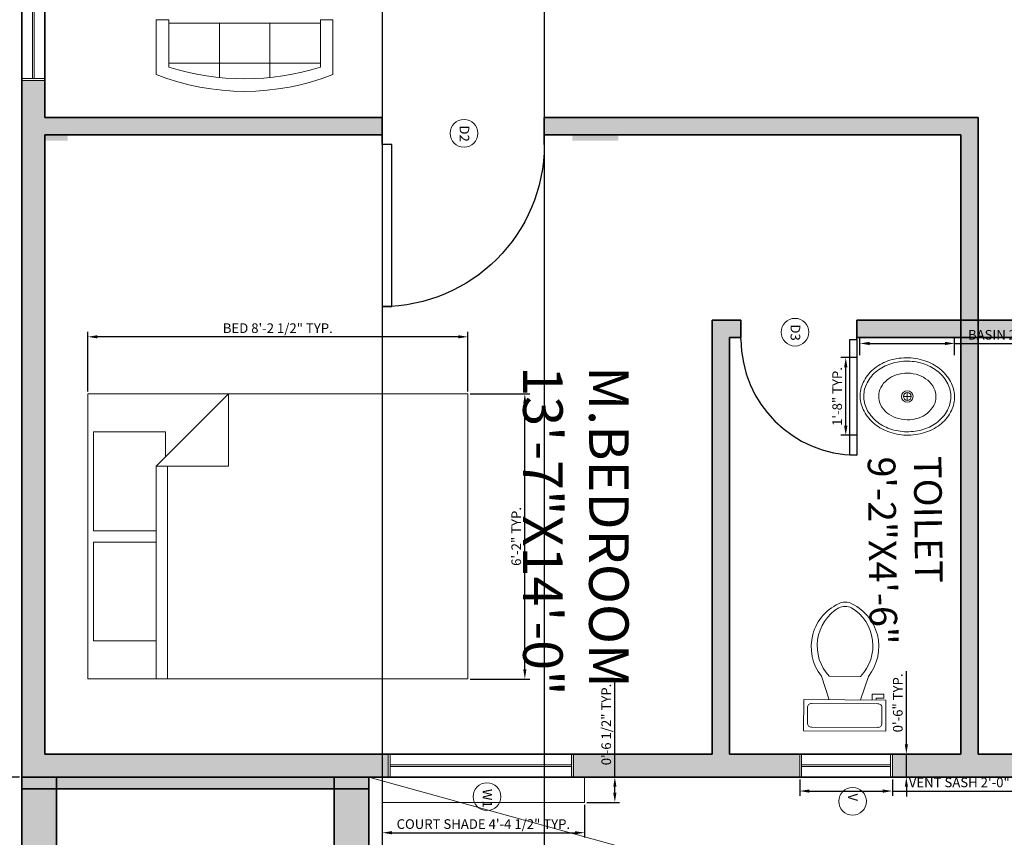
# Model space of a CAD drawing. Units: inches. Extents: x 7028582 to 7030319, y 63109697 to 63111305.
# Tile 14 of 18: x 7029748 to 7030003, y 63110530 to 63110742. Entities that reach past the tile are written whole.
import ezdxf

# ---------------------------------------------------------------- set-up
doc = ezdxf.new("R2010")
doc.units = ezdxf.units.IN
for name, color, linetype, lineweight in [('A-AREA-IDEN', 7, 'Continuous', 18), ('A-DOOR-IDEN', 20, 'Continuous', 13), ('A-FLOR-FIXT', 9, 'Continuous', 18), ('A-FLOR-OPEN', 7, 'Continuous', 13), ('A-GLAZ-IDEN', 20, 'Continuous', 13), ('A-WALL-PATT', 8, 'Continuous', 13), ('C-ANNO-DIMS', 7, 'Continuous', 18), ('doors', 20, 'Continuous', 25), ('furniture', 9, 'Continuous', 18), ('S-COLS-PATT', 220, 'Continuous', 100), ('walls', 6, 'Continuous', 35), ('WINDOW SHADOW', 9, 'Continuous', 13), ('windows', 5, 'Continuous', 18)]:
    doc.layers.add(name, color=color, linetype=linetype, lineweight=lineweight)
doc.styles.get("Standard").update_dxf_attribs({"font": 'arial.ttf'})
doc.dimstyles.new('ISO-25', dxfattribs={"dimtxt": 2.5, "dimasz": 2.5, "dimexe": 1.25, "dimexo": 0.625, "dimtad": 1, "dimlunit": 4, "dimtxsty": 'Standard', "dimcen": 2.5, "dimadec": 0, "dimazin": 0, "dimtfac": 1, "dimtmove": 0, "dimatfit": 3, "dimfxl": 1, "dimarcsym": 0})

# ---------------------------------------------------------------- blocks, each defined once
blk = doc.blocks.new('*U2')
for p, q in [((0, 0), (0, -5)), ((30, 0), (30, -5))]:
    blk.add_line(p, q)
blk.add_lwpolyline([(0, 0), (0, 30), (1.75, 30), (1.75, 0)], close=True)
blk.add_arc((0, 0), 30, 0, 90)
blk = doc.blocks.new('Toilet - top')
for p, q in [((9.5, -6), (9.5, -2)), ((-10, -8.5), (-8, -8.5)), ((-10, -9.5), (-10, -8.5)), ((-7, -9.5), (-10, -9.5)), ((-8, -8.5), (-8, -8)), ((-7, -8), (-7, -9.5)), ((-4, -8), (-6, -14)), ((4, -8), (6, -14)), ((4, -14), (-4, -14))]:
    blk.add_line(p, q)
blk.add_lwpolyline([(10.5, -8), (10.5, 0), (-10.5, 0), (-10.5, -8)], close=True)
for points in [[(-9.5, -2), (-9.5, -6)], [(8.5, -1), (-8.5, -1)], [(-8.5, -7), (8.5, -7)]]:
    blk.add_lwpolyline(points)
for centre, radius, start, end in [((-8.62, -1.88), 0.884, 81.8699, 188.1301), ((8.62, -1.88), 0.884, 351.8699, 98.1301), ((-8.62, -6.12), 0.884, 171.8699, 278.1301), ((8.62, -6.12), 0.884, 261.8699, 8.1301), ((3.52, -21.58), 12.17, 141.4691, 247.9714), ((4.2, -21.82), 11.33, 136.3677, 238.9468), ((-3.52, -21.58), 12.17, 292.0284, 38.5307), ((-4.2, -21.82), 11.33, 301.053, 43.6321), ((0, -27.88), 4, 245.7318, 294.2682), ((0, -29), 4, 254.8605, 285.1395)]:
    blk.add_arc(centre, radius, start, end)
blk = doc.blocks.new('Sink - Oval top')
for p, q in [((-1, 0), (1, 0)), ((0, 1), (0, -1))]:
    blk.add_line(p, q)
for points in [[(-12.23, 0.39, 0.117634), (-11.46, -3.36, 0.104469), (-8.88, -6.8, 0.090016), (-5.08, -9.07, 0.08192), (-0.32, -10.02, 0.08192), (4.49, -9.38, 0.090016), (8.42, -7.36, 0.104469), (11.22, -4.09, 0.117634), (12.23, -0.39, 0.117634), (11.46, 3.36, 0.104469), (8.88, 6.8, 0.090016), (5.08, 9.07, 0.08192), (0.32, 10.02, 0.08192), (-4.49, 9.38, 0.090016), (-8.42, 7.36, 0.104469), (-11.22, 4.09, 0.117634)], [(-11.29, 0.16, 0.118622), (-10.52, -3.25, 0.104678), (-8.07, -6.36, 0.089562), (-4.54, -8.37, 0.081185), (-0.13, -9.15, 0.081185), (4.3, -8.49, 0.089562), (7.89, -6.58, 0.104678), (10.42, -3.55, 0.118622), (11.29, -0.16, 0.118622), (10.52, 3.25, 0.104678), (8.07, 6.36, 0.089562), (4.54, 8.37, 0.081185), (0.13, 9.15, 0.081185), (-4.3, 8.49, 0.089562), (-7.89, 6.58, 0.104678), (-10.42, 3.55, 0.118622)], [(-7.42, 0.08, 0.118283), (-6.91, -2.17, 0.104607), (-5.29, -4.21, 0.089718), (-2.97, -5.53, 0.081436), (-0.07, -6.04, 0.081436), (2.84, -5.59, 0.089718), (5.2, -4.33, 0.104607), (6.86, -2.32, 0.118283), (7.42, -0.08, 0.118283), (6.91, 2.17, 0.104607), (5.29, 4.21, 0.089718), (2.97, 5.53, 0.081436), (0.07, 6.04, 0.081436), (-2.84, 5.59, 0.089718), (-5.2, 4.33, 0.104607), (-6.86, 2.32, 0.118283)]]:
    blk.add_lwpolyline(points, format="xyb", close=True)
for radius in [1.5, 1]:
    blk.add_circle((0, 0), radius)
blk = doc.blocks.new('Bed - Queen')
for p, q in [((0, -80.00003), (0, 0)), ((0, 0), (59.99999, 0)), ((59.99999, 0), (59.99999, -80.00003)), ((7.99999, -1.2), (28.79998, -1.2)), ((7.99999, -14.4), (7.99999, -1.2)), ((28.79998, -1.2), (28.79998, -14.4)), ((31.19999, -1.2), (51.99999, -1.2)), ((31.19999, -14.4), (31.19999, -1.2)), ((51.99999, -1.2), (51.99999, -16.4)), ((0, -14.4), (44.8, -14.4)), ((59.99999, -29.6), (44.8, -14.4)), ((44.8, -14.4), (44.8, -29.6)), ((51.99999, -16.4), (46.79936, -16.4)), ((44.8, -16.8), (0, -16.8)), ((44.8, -29.6), (59.99999, -29.6)), ((59.99999, -80.00003), (0, -80.00003))]:
    blk.add_line(p, q)
blk = doc.blocks.new('Sofa - Roundback 7 ft.')
for p, q in [((-12.00002, -32.4421), (-12.00003, -6.5971)), ((11.99997, -32.4421), (11.99998, -6.5971)), ((-36.000027, -34), (-36.000027, -11.4696)), ((-35.999844, -13.3819), (35.9998, -13.3819)), ((35.99998, -34), (35.99998, -11.4696)), ((-36.000027, -32.4421), (35.99998, -32.4421))]:
    blk.add_line(p, q)
for points in [[(-36.000027, -34), (-42.000027, -34), (-42.000027, -8)], [(41.99998, -8), (41.99998, -34), (35.99998, -34)]]:
    blk.add_lwpolyline(points)
for centre, radius, start, end in [((0, -114.25), 114.25, 68.43141, 111.5686), ((-0.00001, -127.1968), 121.1968, 72.72033, 107.2797)]:
    blk.add_arc(centre, radius, start, end)
blk = doc.blocks.new('WIN-SASH-24')
for p, q in [((24.05, 6), (0, 6)), ((0.5, 6), (0.5, 0)), ((23.55, 0), (23.55, 6)), ((23.55, 3.2), (0.5, 3.2)), ((23.55, 2.8), (0.5, 2.8)), ((0, 0), (24.05, 0))]:
    blk.add_line(p, q)
blk = doc.blocks.new('WIN-SASH-48')
for p, q in [((48.05, 6), (0, 6)), ((0.5, 6), (0.5, 0)), ((47.55, 0), (47.55, 6)), ((47.55, 3.2), (0.5, 3.2)), ((47.55, 2.8), (0.5, 2.8)), ((0, 0), (48.05, 0))]:
    blk.add_line(p, q)
blk = doc.blocks.new('WINDOW-SHADE-COURT-52')
for p, q in [((0, 0), (0, 6.54)), ((52.45, 6.54), (52.45, 0)), ((52.45, 0), (0, 0))]:
    blk.add_line(p, q)
blk = doc.blocks.new('TAG-D2-MT-R')
blk.add_circle((3.58, 3.58), 3.58)
at = {"insert": (4.93, 5.6), "char_height": 2.5, "attachment_point": 1, "rotation": 270}
blk.add_mtext_dynamic_manual_height_columns('D2', width=2.5021, gutter_width=12.5, heights=[0], dxfattribs=at)
blk = doc.blocks.new('TAG-D3-MT-R')
blk.add_circle((3.58, 3.58), 3.58)
at = {"insert": (4.93, 5.6), "char_height": 2.5, "attachment_point": 1, "rotation": 270}
blk.add_mtext_dynamic_manual_height_columns('D3', width=2.5021, gutter_width=12.5, heights=[0], dxfattribs=at)
blk = doc.blocks.new('TAG-V-MT-R')
blk.add_circle((3.58, 3.58), 3.58)
at = {"insert": (4.93, 5.6), "char_height": 2.5, "attachment_point": 1, "rotation": 270}
blk.add_mtext_dynamic_manual_height_columns('V', width=2.5021, gutter_width=12.5, heights=[0], dxfattribs=at)
blk = doc.blocks.new('TAG-W1-MT-R')
blk.add_circle((3.58, 3.58), 3.58)
at = {"insert": (4.93, 5.6), "char_height": 2.5, "attachment_point": 1, "rotation": 270}
blk.add_mtext_dynamic_manual_height_columns('W1', width=2.5021, gutter_width=12.5, heights=[0], dxfattribs=at)
blk = doc.blocks.new('*D55')
at = {"layer": 'C-ANNO-DIMS', "color": 0, "lineweight": -2, "transparency": 16777216}
for p, q in [((7029949.93, 63110544.93), (7029949.93, 63110540.7)), ((7029973.98, 63110544.93), (7029973.98, 63110540.7)), ((7029952.43, 63110541.95), (7029971.48, 63110541.95)), ((7029973.98, 63110541.95), (7030013.86, 63110541.95))]:
    blk.add_line(p, q, dxfattribs=at)
at = {"layer": 'C-ANNO-DIMS', "color": 0, "lineweight": 100, "transparency": 16777216}
for points in [[(7029952.43, 63110542.37), (7029952.43, 63110541.53), (7029949.93, 63110541.95)], [(7029971.48, 63110542.37), (7029971.48, 63110541.53), (7029973.98, 63110541.95)]]:
    blk.add_solid(points, dxfattribs=at)
at = {"layer": 'Defpoints', "color": 0, "lineweight": 100, "transparency": 16777216}
for p in [(7029949.93, 63110545.56), (7029973.98, 63110545.56), (7029973.98, 63110541.95)]:
    blk.add_point(p, dxfattribs=at)
at = {"layer": 'C-ANNO-DIMS', "color": 0, "transparency": 16777216, "insert": (7029995.17, 63110543.87), "char_height": 2.5, "attachment_point": 5}
blk.add_mtext('VENT SASH 2\'-0" TYP.', dxfattribs=at)
blk = doc.blocks.new('*D56')
at = {"layer": 'C-ANNO-DIMS', "color": 0, "lineweight": -2, "transparency": 16777216}
for p, q in [((7029977.59, 63110554.06), (7029977.59, 63110573.05)), ((7029974.6, 63110551.56), (7029978.84, 63110551.56)), ((7029977.59, 63110545.56), (7029977.59, 63110551.56)), ((7029974.6, 63110545.56), (7029978.84, 63110545.56)), ((7029977.59, 63110543.06), (7029977.59, 63110540.56))]:
    blk.add_line(p, q, dxfattribs=at)
at = {"layer": 'C-ANNO-DIMS', "color": 0, "lineweight": 100, "transparency": 16777216}
for points in [[(7029977.17, 63110554.06), (7029978, 63110554.06), (7029977.59, 63110551.56)], [(7029977.17, 63110543.06), (7029978, 63110543.06), (7029977.59, 63110545.56)]]:
    blk.add_solid(points, dxfattribs=at)
at = {"layer": 'Defpoints', "color": 0, "lineweight": 100, "transparency": 16777216}
for p in [(7029973.98, 63110551.56), (7029977.59, 63110551.56), (7029973.98, 63110545.56)]:
    blk.add_point(p, dxfattribs=at)
at = {"layer": 'C-ANNO-DIMS', "color": 0, "transparency": 16777216, "insert": (7029975.69, 63110564.8), "char_height": 2.5, "attachment_point": 5, "rotation": 90}
blk.add_mtext('0\'-6" TYP.', dxfattribs=at)
blk = doc.blocks.new('*D61')
at = {"layer": 'C-ANNO-DIMS', "color": 0, "lineweight": -2, "transparency": 16777216}
for p, q in [((7029965.55, 63110654.94), (7029965.55, 63110659.24)), ((7029990.1, 63110654.94), (7029990.1, 63110659.24)), ((7029968.05, 63110657.99), (7029987.6, 63110657.99)), ((7029990.1, 63110657.99), (7030026.26, 63110657.99))]:
    blk.add_line(p, q, dxfattribs=at)
at = {"layer": 'C-ANNO-DIMS', "color": 0, "lineweight": 100, "transparency": 16777216}
for points in [[(7029968.05, 63110658.41), (7029968.05, 63110657.58), (7029965.55, 63110657.99)], [(7029987.6, 63110658.41), (7029987.6, 63110657.58), (7029990.1, 63110657.99)]]:
    blk.add_solid(points, dxfattribs=at)
at = {"layer": 'Defpoints', "color": 0, "lineweight": 100, "transparency": 16777216}
for p in [(7029990.1, 63110657.99), (7029965.55, 63110654.31), (7029990.1, 63110654.31)]:
    blk.add_point(p, dxfattribs=at)
at = {"layer": 'C-ANNO-DIMS', "color": 0, "transparency": 16777216, "insert": (7030009.43, 63110659.91), "char_height": 2.5, "attachment_point": 5}
blk.add_mtext('BASIN 2\'-0 1/2" TYP.', dxfattribs=at)
blk = doc.blocks.new('*D62')
at = {"layer": 'C-ANNO-DIMS', "color": 0, "lineweight": -2, "transparency": 16777216}
for p, q in [((7029964.93, 63110654.31), (7029960.62, 63110654.31)), ((7029961.87, 63110636.67), (7029961.87, 63110651.81)), ((7029964.93, 63110634.17), (7029960.62, 63110634.17))]:
    blk.add_line(p, q, dxfattribs=at)
at = {"layer": 'C-ANNO-DIMS', "color": 0, "lineweight": 100, "transparency": 16777216}
for points in [[(7029961.45, 63110651.81), (7029962.29, 63110651.81), (7029961.87, 63110654.31)], [(7029961.45, 63110636.67), (7029962.29, 63110636.67), (7029961.87, 63110634.17)]]:
    blk.add_solid(points, dxfattribs=at)
at = {"layer": 'Defpoints', "color": 0, "lineweight": 100, "transparency": 16777216}
for p in [(7029961.87, 63110654.31), (7029965.55, 63110654.31), (7029965.55, 63110634.17)]:
    blk.add_point(p, dxfattribs=at)
at = {"layer": 'C-ANNO-DIMS', "color": 0, "transparency": 16777216, "insert": (7029959.97, 63110644.24), "char_height": 2.5, "attachment_point": 5, "rotation": 90}
blk.add_mtext('1\'-8" TYP.', dxfattribs=at)
blk = doc.blocks.new('*D65')
at = {"layer": 'C-ANNO-DIMS', "color": 0, "lineweight": -2, "transparency": 16777216}
for p, q in [((7029765.3, 63110645.55), (7029765.3, 63110660.96)), ((7029861.37, 63110659.71), (7029767.8, 63110659.71)), ((7029863.87, 63110645.55), (7029863.87, 63110660.96))]:
    blk.add_line(p, q, dxfattribs=at)
at = {"layer": 'C-ANNO-DIMS', "color": 0, "lineweight": 100, "transparency": 16777216}
for points in [[(7029767.8, 63110660.13), (7029767.8, 63110659.3), (7029765.3, 63110659.71)], [(7029861.37, 63110660.13), (7029861.37, 63110659.3), (7029863.87, 63110659.71)]]:
    blk.add_solid(points, dxfattribs=at)
at = {"layer": 'Defpoints', "color": 0, "lineweight": 100, "transparency": 16777216}
for p in [(7029765.3, 63110659.71), (7029765.3, 63110644.93), (7029863.87, 63110644.93)]:
    blk.add_point(p, dxfattribs=at)
at = {"layer": 'C-ANNO-DIMS', "color": 0, "transparency": 16777216, "insert": (7029814.59, 63110661.63), "char_height": 2.5, "attachment_point": 5}
blk.add_mtext('BED 8\'-2 1/2" TYP.', dxfattribs=at)
blk = doc.blocks.new('*D66')
at = {"layer": 'C-ANNO-DIMS', "color": 0, "lineweight": -2, "transparency": 16777216}
for p, q in [((7029864.5, 63110644.93), (7029879.91, 63110644.93)), ((7029878.66, 63110573.5), (7029878.66, 63110642.43)), ((7029864.5, 63110571), (7029879.91, 63110571))]:
    blk.add_line(p, q, dxfattribs=at)
at = {"layer": 'C-ANNO-DIMS', "color": 0, "lineweight": 100, "transparency": 16777216}
for points in [[(7029878.24, 63110642.43), (7029879.07, 63110642.43), (7029878.66, 63110644.93)], [(7029878.24, 63110573.5), (7029879.07, 63110573.5), (7029878.66, 63110571)]]:
    blk.add_solid(points, dxfattribs=at)
at = {"layer": 'Defpoints', "color": 0, "lineweight": 100, "transparency": 16777216}
for p in [(7029863.87, 63110644.93), (7029878.66, 63110644.93), (7029863.87, 63110571)]:
    blk.add_point(p, dxfattribs=at)
at = {"layer": 'C-ANNO-DIMS', "color": 0, "transparency": 16777216, "insert": (7029876.75, 63110607.96), "char_height": 2.5, "attachment_point": 5, "rotation": 90}
blk.add_mtext('6\'-2" TYP.', dxfattribs=at)
blk = doc.blocks.new('*D95')
at = {"layer": 'C-ANNO-DIMS', "color": 0, "lineweight": -2, "transparency": 16777216}
for p, q in [((7029841.67, 63110538.39), (7029841.67, 63110529.9)), ((7029894.13, 63110538.39), (7029894.13, 63110529.9)), ((7029844.17, 63110531.15), (7029891.63, 63110531.15))]:
    blk.add_line(p, q, dxfattribs=at)
at = {"layer": 'C-ANNO-DIMS', "color": 0, "lineweight": 100, "transparency": 16777216}
for points in [[(7029844.17, 63110531.56), (7029844.17, 63110530.73), (7029841.67, 63110531.15)], [(7029891.63, 63110531.56), (7029891.63, 63110530.73), (7029894.13, 63110531.15)]]:
    blk.add_solid(points, dxfattribs=at)
at = {"layer": 'Defpoints', "color": 0, "lineweight": 100, "transparency": 16777216}
for p in [(7029841.67, 63110539.02), (7029894.13, 63110539.02), (7029894.13, 63110531.15)]:
    blk.add_point(p, dxfattribs=at)
at = {"layer": 'C-ANNO-DIMS', "color": 0, "transparency": 16777216, "insert": (7029867.9, 63110533.07), "char_height": 2.5, "attachment_point": 5}
blk.add_mtext('COURT SHADE 4\'-4 1/2" TYP.', dxfattribs=at)
blk = doc.blocks.new('*D96')
at = {"layer": 'C-ANNO-DIMS', "color": 0, "lineweight": -2, "transparency": 16777216}
for p, q in [((7029901.99, 63110545.56), (7029901.99, 63110570.37)), ((7029894.75, 63110545.56), (7029903.24, 63110545.56)), ((7029901.99, 63110541.52), (7029901.99, 63110543.06)), ((7029894.75, 63110539.02), (7029903.24, 63110539.02))]:
    blk.add_line(p, q, dxfattribs=at)
at = {"layer": 'C-ANNO-DIMS', "color": 0, "lineweight": 100, "transparency": 16777216}
for points in [[(7029901.58, 63110543.06), (7029902.41, 63110543.06), (7029901.99, 63110545.56)], [(7029901.58, 63110541.52), (7029902.41, 63110541.52), (7029901.99, 63110539.02)]]:
    blk.add_solid(points, dxfattribs=at)
at = {"layer": 'Defpoints', "color": 0, "lineweight": 100, "transparency": 16777216}
for p in [(7029894.13, 63110545.56), (7029901.99, 63110545.56), (7029894.13, 63110539.02)]:
    blk.add_point(p, dxfattribs=at)
at = {"layer": 'C-ANNO-DIMS', "color": 0, "transparency": 16777216, "insert": (7029900.08, 63110559.21), "char_height": 2.5, "attachment_point": 5, "rotation": 90}
blk.add_mtext('0\'-6 1/2" TYP.', dxfattribs=at)
blk = doc.blocks.new('*D105')
at = {"layer": 'C-ANNO-DIMS', "color": 0, "lineweight": -2, "transparency": 16777216}
for p, q in [((7029841.68, 63110859.93), (7029841.68, 63109697.14)), ((7029883.68, 63110859.93), (7029883.68, 63109697.14)), ((7029844.18, 63109698.39), (7029881.18, 63109698.39))]:
    blk.add_line(p, q, dxfattribs=at)
at = {"layer": 'C-ANNO-DIMS', "color": 0, "lineweight": 100, "transparency": 16777216}
for points in [[(7029844.18, 63109698.8), (7029844.18, 63109697.97), (7029841.68, 63109698.39)], [(7029881.18, 63109698.8), (7029881.18, 63109697.97), (7029883.68, 63109698.39)]]:
    blk.add_solid(points, dxfattribs=at)
at = {"layer": 'Defpoints', "color": 0, "lineweight": 100, "transparency": 16777216}
for p in [(7029841.68, 63110860.56), (7029883.68, 63110860.56), (7029883.68, 63109698.39)]:
    blk.add_point(p, dxfattribs=at)
at = {"layer": 'C-ANNO-DIMS', "color": 0, "transparency": 16777216, "insert": (7029862.68, 63109700.29), "char_height": 2.5, "attachment_point": 5}
blk.add_mtext('3\'-6"', dxfattribs=at)
blk = doc.blocks.new('*D112')
at = {"layer": 'C-ANNO-DIMS', "color": 0, "lineweight": -2, "transparency": 16777216}
for p, q in [((7029747.58, 63111033.06), (7028586.23, 63111033.06)), ((7028587.48, 63111030.56), (7028587.48, 63110548.06)), ((7029747.58, 63110545.56), (7028586.23, 63110545.56))]:
    blk.add_line(p, q, dxfattribs=at)
at = {"layer": 'C-ANNO-DIMS', "color": 0, "lineweight": 100, "transparency": 16777216}
for points in [[(7028587.06, 63111030.56), (7028587.89, 63111030.56), (7028587.48, 63111033.06)], [(7028587.06, 63110548.06), (7028587.89, 63110548.06), (7028587.48, 63110545.56)]]:
    blk.add_solid(points, dxfattribs=at)
at = {"layer": 'Defpoints', "color": 0, "lineweight": 100, "transparency": 16777216}
for p in [(7029748.21, 63111033.06), (7028587.48, 63110545.56), (7029748.21, 63110545.56)]:
    blk.add_point(p, dxfattribs=at)
at = {"layer": 'C-ANNO-DIMS', "color": 0, "transparency": 16777216, "insert": (7028585.56, 63110789.31), "char_height": 2.5, "attachment_point": 5, "rotation": 90}
blk.add_mtext('40\'-7 1/2"', dxfattribs=at)

msp = doc.modelspace()

# ---------------------------------------------------------------- hatches: boundary and pattern name
at = {"layer": 'A-WALL-PATT'}
h = msp.add_hatch(color=256, dxfattribs=at)
h.dxf.hatch_style = 1
h.paths.add_polyline_path([(7029841.685, 63110716.557), (7029754.205, 63110716.557), (7029754.205, 63110726.137), (7029748.205, 63110726.137), (7029748.205, 63110545.557), (7029837.679, 63110545.557), (7029837.679, 63110551.557), (7029754.205, 63110551.557), (7029754.205, 63110712.057), (7029841.685, 63110712.057)])
h = msp.add_hatch(color=256, dxfattribs=at)
h.dxf.hatch_style = 1
h.paths.add_polyline_path([(7029843.226, 63110551.557), (7029754.205, 63110551.557), (7029754.205, 63110712.057), (7029841.685, 63110712.057), (7029841.685, 63110716.557), (7029754.205, 63110716.557), (7029754.205, 63110726.137), (7029748.205, 63110726.137), (7029748.205, 63110545.557), (7029843.226, 63110545.557)])
h = msp.add_hatch(color=256, dxfattribs=at)
h.dxf.hatch_style = 1
h.paths.add_polyline_path([(7029996.205, 63110716.557), (7029883.685, 63110716.557), (7029883.685, 63110712.057), (7029991.705, 63110712.057), (7029991.705, 63110664.057), (7029996.205, 63110664.057)])
h = msp.add_hatch(color=256, dxfattribs=at)
h.dxf.hatch_style = 1
h.paths.add_polyline_path([(7029949.931, 63110551.557), (7029931.705, 63110551.557), (7029931.705, 63110659.557), (7029934.705, 63110659.557), (7029934.705, 63110664.057), (7029927.205, 63110664.057), (7029927.205, 63110551.557), (7029891.274, 63110551.557), (7029891.274, 63110545.557), (7029949.931, 63110545.557)])
h = msp.add_hatch(color=256, dxfattribs=at)
h.dxf.hatch_style = 1
h.paths.add_polyline_path([(7029991.705, 63110664.057), (7029964.705, 63110664.057), (7029964.705, 63110659.557), (7029991.705, 63110659.557)])
h = msp.add_hatch(color=256, dxfattribs=at)
h.dxf.hatch_style = 1
h.paths.add_polyline_path([(7029996.205, 63110664.057), (7029991.705, 63110664.057), (7029991.705, 63110659.557), (7029996.205, 63110659.557)])
h = msp.add_hatch(color=256, dxfattribs=at)
h.dxf.hatch_style = 1
h.paths.add_polyline_path([(7030049.705, 63110664.057), (7029996.205, 63110664.057), (7029996.205, 63110659.557), (7030045.205, 63110659.557), (7030045.205, 63110656.557), (7030049.705, 63110656.557)])
h = msp.add_hatch(color=256, dxfattribs=at)
h.dxf.hatch_style = 1
h.paths.add_polyline_path([(7029996.205, 63110659.557), (7029991.705, 63110659.557), (7029991.705, 63110551.557), (7029973.979, 63110551.557), (7029973.979, 63110545.557), (7030008.697, 63110545.557), (7030008.697, 63110551.557), (7029996.205, 63110551.557)])
h = msp.add_hatch(color=256, dxfattribs=at)
h.dxf.hatch_style = 1
h.paths.add_polyline_path([(7029757.205, 63110545.557), (7029748.205, 63110545.557), (7029748.205, 63110542.557), (7029757.205, 63110542.557)])
h = msp.add_hatch(color=256, dxfattribs=at)
h.dxf.hatch_style = 1
h.paths.add_polyline_path([(7029829.205, 63110545.557), (7029757.205, 63110545.557), (7029757.205, 63110542.557), (7029829.205, 63110542.557)])
h = msp.add_hatch(color=256, dxfattribs=at)
h.dxf.hatch_style = 1
h.paths.add_polyline_path([(7029838.205, 63110545.557), (7029829.205, 63110545.557), (7029829.205, 63110542.557), (7029838.205, 63110542.557)])
h = msp.add_hatch(color=256, dxfattribs=at)
h.dxf.hatch_style = 1
h.paths.add_polyline_path([(7029757.205, 63110542.557), (7029748.205, 63110542.557), (7029748.205, 63110457.057), (7029757.205, 63110457.057)])
h = msp.add_hatch(color=256, dxfattribs=at)
h.dxf.hatch_style = 1
h.paths.add_polyline_path([(7029838.205, 63110542.557), (7029829.205, 63110542.557), (7029829.205, 63110457.057), (7029838.205, 63110457.057)])
at = {"layer": 'S-COLS-PATT'}
h = msp.add_hatch(color=256, dxfattribs=at)
h.dxf.hatch_style = 1
h.paths.add_polyline_path([(7029760.108, 63110716.557), (7029748.205, 63110716.557), (7029748.205, 63110710.557), (7029760.108, 63110710.557)])
h = msp.add_hatch(color=256, dxfattribs=at)
h.dxf.hatch_style = 1
h.paths.add_polyline_path([(7029902.915, 63110716.557), (7029891, 63110716.557), (7029891, 63110710.557), (7029902.915, 63110710.557)])
h = msp.add_hatch(color=256, dxfattribs=at)
h.dxf.hatch_style = 1
h.paths.add_polyline_path([(7029760.108, 63110551.607), (7029748.205, 63110551.607), (7029748.205, 63110545.607), (7029760.108, 63110545.607)])
h = msp.add_hatch(color=256, dxfattribs=at)
h.dxf.hatch_style = 1
h.paths.add_polyline_path([(7029902.915, 63110551.607), (7029891, 63110551.607), (7029891, 63110545.607), (7029902.915, 63110545.607)])

# ---------------------------------------------------------------- linework, layer by layer
at = {"layer": 'A-FLOR-OPEN'}
msp.add_line((7030169.705, 63110454.057), (7029838.205, 63110545.557), dxfattribs=at)
at = {"layer": 'walls'}
for p, q in [((7029748.205, 63110545.557), (7029748.205, 63110809.557)), ((7029754.205, 63110716.557), (7029754.205, 63110809.557)), ((7029841.685, 63110716.557), (7029754.205, 63110716.557)), ((7029841.685, 63110712.057), (7029841.685, 63110716.557)), ((7029883.685, 63110716.557), (7029883.685, 63110712.057)), ((7029996.205, 63110716.557), (7029883.685, 63110716.557)), ((7029996.205, 63110551.557), (7029996.205, 63110716.557)), ((7029754.205, 63110551.557), (7029754.205, 63110712.057)), ((7029841.685, 63110712.057), (7029754.205, 63110712.057)), ((7029991.705, 63110712.057), (7029883.685, 63110712.057)), ((7029991.705, 63110551.557), (7029991.705, 63110712.057)), ((7029927.205, 63110551.557), (7029927.205, 63110664.057)), ((7029934.705, 63110664.057), (7029927.205, 63110664.057)), ((7029934.705, 63110659.557), (7029934.705, 63110664.057)), ((7030049.705, 63110664.057), (7029964.705, 63110664.057)), ((7029964.705, 63110664.057), (7029964.705, 63110659.557)), ((7029931.705, 63110551.557), (7029931.705, 63110659.557)), ((7029931.705, 63110659.557), (7029934.705, 63110659.557)), ((7029934.705, 63110659.557), (7029931.705, 63110659.557)), ((7030045.205, 63110659.557), (7029964.705, 63110659.557)), ((7029927.205, 63110551.557), (7029754.205, 63110551.557)), ((7029991.705, 63110551.557), (7029931.705, 63110551.557)), ((7030045.205, 63110551.557), (7029996.205, 63110551.557)), ((7030175.705, 63110545.557), (7029748.205, 63110545.557)), ((7029748.205, 63110545.557), (7029748.205, 63110542.557)), ((7029757.205, 63110545.557), (7029757.205, 63110454.057)), ((7029829.205, 63110454.057), (7029829.205, 63110545.557)), ((7029838.205, 63110454.057), (7029838.205, 63110545.557)), ((7029748.205, 63110542.557), (7029757.205, 63110542.557)), ((7029748.205, 63110542.557), (7029748.205, 63110457.057)), ((7029757.205, 63110542.557), (7029829.205, 63110542.557)), ((7029829.205, 63110542.557), (7029838.205, 63110542.557))]:
    msp.add_line(p, q, dxfattribs=at)
at = {"layer": 'windows'}
for p, q in [((7029748.205, 63110726.137), (7029754.205, 63110726.137)), ((7029843.226, 63110551.557), (7029843.226, 63110545.557)), ((7029891.274, 63110545.557), (7029891.274, 63110551.557)), ((7029949.931, 63110551.557), (7029949.931, 63110545.557)), ((7029973.979, 63110545.557), (7029973.979, 63110551.557))]:
    msp.add_line(p, q, dxfattribs=at)

# ---------------------------------------------------------------- block references
at = {"layer": 'A-DOOR-IDEN'}
for name, p in [('TAG-D2-MT-R', (7029859.301, 63110708.893)), ('TAG-D3-MT-R', (7029945.138, 63110657.328))]:
    msp.add_blockref(name, p, dxfattribs=at)
at = {"layer": 'A-FLOR-FIXT'}
msp.add_blockref('Sink - Oval top', (7029977.829, 63110644.243), dxfattribs=at)
at = {"layer": 'A-FLOR-FIXT', "xscale": 1.013555723357934, "yscale": 1.013555723357934, "zscale": 1.013555723357934, "rotation": 179.7253796204469}
msp.add_blockref('Toilet - top', (7029961.58, 63110557.497), dxfattribs=at)
at = {"layer": 'A-GLAZ-IDEN'}
for name, p in [('TAG-W1-MT-R', (7029865.247, 63110536.914)), ('TAG-V-MT-R', (7029960.057, 63110535.713))]:
    msp.add_blockref(name, p, dxfattribs=at)
at = {"layer": 'doors', "xscale": -1.399999999999999, "yscale": 1.399999999999999, "zscale": 1.399999999999999, "rotation": 180}
msp.add_blockref('*U2', (7029841.685, 63110709.557), dxfattribs=at)
at = {"layer": 'doors', "rotation": 180}
msp.add_blockref('*U2', (7029964.705, 63110659.057), dxfattribs=at)
at = {"layer": 'furniture'}
for name, p, xscale, yscale, zscale, rotation in [('Sofa - Roundback 7 ft.', (7029805.982, 63110723.346), 0.5455524879488546, 0.5455524879488546, 0.5455524879488546, 180), ('Bed - Queen', (7029765.303, 63110571.002), 1.232093012797833, 1.232093012797833, 1.232093012797833, 89.99999999999999)]:
    msp.add_blockref(name, p, dxfattribs=dict(at, xscale=xscale, yscale=yscale, zscale=zscale, rotation=rotation))
at = {"layer": 'WINDOW SHADOW'}
msp.add_blockref('WINDOW-SHADE-COURT-52', (7029841.671, 63110539.016), dxfattribs=at)
at = {"layer": 'windows', "rotation": 89.99999995093432}
msp.add_blockref('WIN-SASH-24', (7029754.205, 63110726.137), dxfattribs=at)
at = {"layer": 'windows'}
for name, p in [('WIN-SASH-48', (7029843.226, 63110545.557)), ('WIN-SASH-24', (7029949.931, 63110545.557))]:
    msp.add_blockref(name, p, dxfattribs=at)

# ---------------------------------------------------------------- texts
at = {"layer": 'A-AREA-IDEN', "attachment_point": 1}
for s, width, gutter_width, insert, char_height, rotation in [('M.BEDROOM\\P13\'-7"X14\'-0"', 82.04322, 51.315, (7029905.577, 63110652.083), 10.26307, 270), ('TOILET\\P9\'-2"X4\'-6"', 42.97461, 35.821, (7029986.665, 63110628.835), 7.16426, 270.6464)]:
    msp.add_mtext_dynamic_manual_height_columns(s, width=width, gutter_width=gutter_width, heights=[0], dxfattribs=dict(at, insert=insert, char_height=char_height, rotation=rotation))

# ---------------------------------------------------------------- dimensions: what is measured, and where the dimension line sits
at = {"layer": 'C-ANNO-DIMS'}
dim = msp.add_linear_dim(base=(7028587.475, 63110545.557), p1=(7029748.205, 63111033.057), p2=(7029748.205, 63110545.557), angle=90, dimstyle='ISO-25', override={"dimdec": 1, "dimlfac": 1, "dimrnd": 0, "dimzin": 1, "dimdsep": 46, "dimlunit": 4, "dimfrac": 2}, dxfattribs=at)
dim.commit()
dim.dimension.update_dxf_attribs({"geometry": '*D112', "text_midpoint": (7028585.558, 63110789.307)})
dim = msp.add_linear_dim(base=(7029883.685, 63109698.385), p1=(7029841.685, 63110860.557), p2=(7029883.685, 63110860.557), dimstyle='ISO-25', override={"dimdec": 1, "dimlfac": 1, "dimrnd": 0, "dimzin": 1, "dimdsep": 46, "dimlunit": 4, "dimfrac": 2}, dxfattribs=at)
dim.commit()
dim.dimension.update_dxf_attribs({"geometry": '*D105', "text_midpoint": (7029862.685, 63109700.288)})
for base, p1, p2, angle, text, picture, middle in [((7029765.303, 63110659.713), (7029863.87, 63110644.928), (7029765.303, 63110644.928), 180, 'BED <> TYP.', '*D65', (7029814.586, 63110661.63)), ((7029961.871, 63110654.311), (7029965.553, 63110634.174), (7029965.553, 63110654.311), 90, '<> TYP.', '*D62', (7029959.969, 63110644.243)), ((7029878.655, 63110644.928), (7029863.87, 63110571.002), (7029863.87, 63110644.928), 90, '<> TYP.', '*D66', (7029876.754, 63110607.965)), ((7029977.587, 63110551.557), (7029973.979, 63110545.557), (7029973.979, 63110551.557), 90, '<> TYP.', '*D56', (7029975.685, 63110564.801)), ((7029901.994, 63110545.557), (7029894.126, 63110539.016), (7029894.126, 63110545.557), 90, '<> TYP.', '*D96', (7029900.076, 63110559.214))]:
    dim = msp.add_linear_dim(base=base, p1=p1, p2=p2, angle=angle, text=text, dimstyle='ISO-25', override={"dimdec": 1, "dimlfac": 1, "dimrnd": 0, "dimzin": 1, "dimdsep": 46, "dimlunit": 4, "dimfrac": 2}, dxfattribs=at)
    dim.commit()
    dim.dimension.update_dxf_attribs({"geometry": picture, "text_midpoint": middle})
for base, p1, p2, text, picture, middle in [((7029990.104, 63110657.993), (7029965.553, 63110654.311), (7029990.104, 63110654.311), 'BASIN <> TYP.', '*D61', (7030009.432, 63110659.911)), ((7029973.979, 63110541.949), (7029949.931, 63110545.557), (7029973.979, 63110545.557), 'VENT SASH <> TYP.', '*D55', (7029995.171, 63110543.867)), ((7029894.126, 63110531.148), (7029841.671, 63110539.016), (7029894.126, 63110539.016), 'COURT SHADE <> TYP.', '*D95', (7029867.898, 63110533.067))]:
    dim = msp.add_linear_dim(base=base, p1=p1, p2=p2, text=text, dimstyle='ISO-25', override={"dimdec": 1, "dimlfac": 1, "dimrnd": 0, "dimzin": 1, "dimdsep": 46, "dimlunit": 4, "dimfrac": 2}, dxfattribs=at)
    dim.commit()
    dim.dimension.update_dxf_attribs({"geometry": picture, "text_midpoint": middle})

doc.saveas('drawing.dxf')
